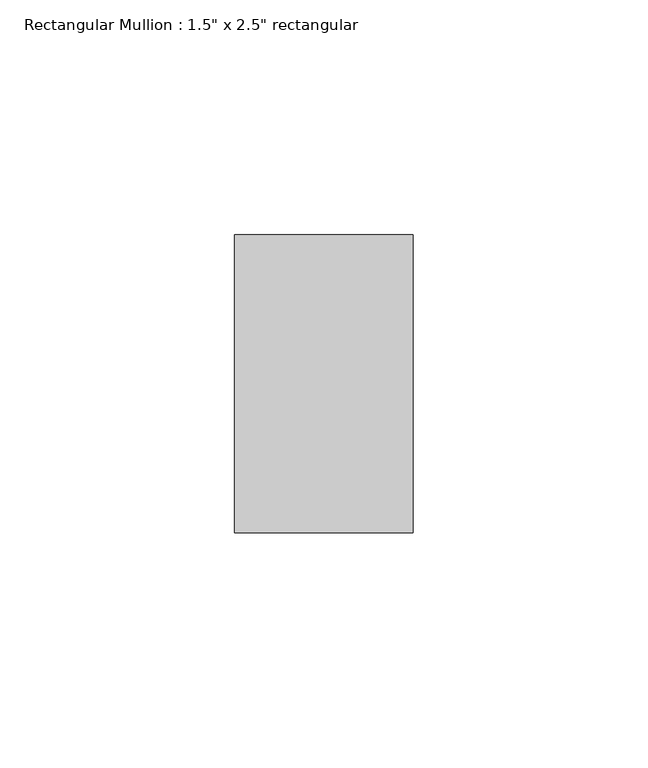
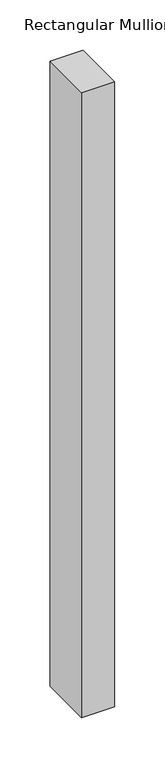
"""IFC4 building model written with IfcOpenShell, lengths in millimetres: member geometry."""

from ifc_helpers import new_model, si_unit, frame, origin, place, context, project, spatial, polyline, outline, extrude, source, transform, mapped, element, save


def member_1d97dc70(model_context):
    return source(origin(), model_context, "Body", "SweptSolid", [
        extrude(outline(polyline([(0.0, 31.75), (0.0, -31.75), (-38.1, -31.75), (-38.1, 31.75), (0.0, 31.75)])), frame((0.0, 0.0, -762.0), z_axis=(0.0, 0.0, 1.0), x_axis=(1.0, 0.0, 0.0)), (0.0, 0.0, 1.0), 762.0),
    ])


if __name__ == "__main__":
    model = new_model("IFC4")
    model_context = context("Model", 3, world=origin())
    ifc_project = project(units=[si_unit("LENGTHUNIT", "METRE", prefix="MILLI")], contexts=[model_context])
    site = spatial("IfcSite", under=ifc_project)
    building = spatial("IfcBuilding", under=site)
    placement = place(None, origin())
    member_shape = member_1d97dc70(model_context)
    element("IfcMember", 1, ObjectType="Rectangular Mullion : 1.5\" x 2.5\" rectangular", at=placement, inside=building, context=model_context, shape_type="MappedRepresentation", body=[
        mapped(member_shape, transform((0.0, 0.0, 0.0), x_axis=(1.0, 0.0, 0.0), y_axis=(0.0, 1.0, 0.0), z_axis=(0.0, 0.0, 1.0))),
    ])
    save(model, "model.ifc")

# Revit data of these elements
# Type "Rectangular Mullion : 1.5\" x 2.5\" rectangular"
#   built-in parameter 1007304 = 0.208333 (stored number, unit not read)
#   built-in parameter 1007301 = 0.0625 (stored number, unit not read)
#   built-in parameter 1007300 = 0.0625 (stored number, unit not read)
